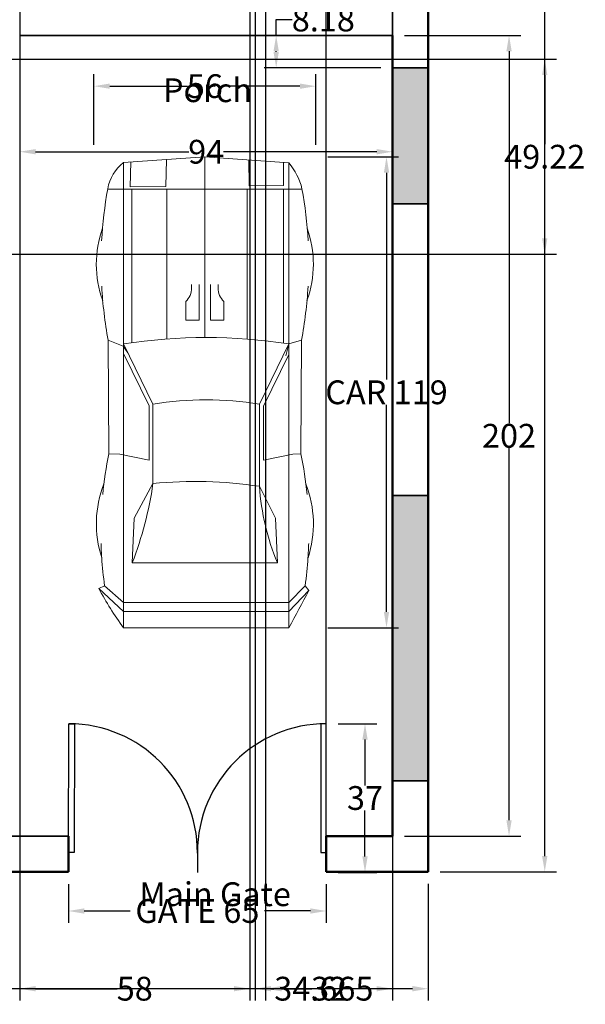
# Model space of a CAD drawing. Units: inches. Extents: x -1285 to -837, y -84 to 552.
# Tile 4 of 10: x -981 to -838, y -84 to 164. Entities that reach past the tile are written whole.
import ezdxf

# ---------------------------------------------------------------- set-up
doc = ezdxf.new("R2010")
doc.units = ezdxf.units.IN
doc.header["$MEASUREMENT"] = 0
for name, color, linetype, lineweight in [('A-ANNO-DIMS', 2, 'Continuous', 18), ('A-ANNO-TEXT', 7, 'Continuous', 18), ('A-AREA-IDEN', 7, 'Continuous', 25), ('A-COLS', 54, 'Continuous', 35), ('A-COLS-PATT', 54, 'Continuous', 13), ('Car', 10, 'Continuous', 18), ('Doors', 34, 'Continuous', 25), ('Inner Wall', 202, 'Continuous', 35), ('Outer Wall', 12, 'Continuous', 50)]:
    doc.layers.add(name, color=color, linetype=linetype, lineweight=lineweight)
doc.styles.get("Standard").update_dxf_attribs({"font": 'arial.ttf'})
doc.dimstyles.get("Standard").update_dxf_attribs({"dimtxt": 6, "dimasz": 4, "dimexe": 3, "dimexo": 3, "dimgap": 0.09, "dimtad": 0, "dimtih": 1, "dimtoh": 1, "dimdec": 1, "dimzin": 0, "dimdsep": 46, "dimlunit": 3, "dimtxsty": 'Standard', "dimcen": 0.09, "dimadec": 0, "dimazin": 0, "dimtfac": 1, "dimtdec": 1, "dimtofl": 0, "dimtmove": 0, "dimatfit": 3, "dimfxl": 1, "dimtolj": 1, "dimtzin": 0, "dimarcsym": 0})

# ---------------------------------------------------------------- blocks, each defined once
blk = doc.blocks.new('Car Top View')
for p, q in [((1583.58, 732.11), (1582.02, 730.88)), ((1587.49, 725.66), (1582.02, 730.88)), ((1590.39, 725.66), (1583.58, 732.11)), ((1454.09, 729.88), (1454.09, 667.25)), ((1504.06, 725.66), (1502.84, 729.72)), ((1502.84, 729.72), (1539.47, 729.51)), ((1539.64, 726.95), (1539.47, 729.51)), ((1443.7, 698.56), (1445.66, 725.66)), ((1595.59, 725.66), (1445.66, 725.66)), ((1504.06, 725.66), (1523.43, 716.14)), ((1507.93, 724.64), (1504.06, 725.66)), ((1507.44, 725.66), (1524.09, 717.48)), ((1541.57, 717.48), (1539.64, 726.95)), ((1587.49, 672.32), (1587.49, 725.66)), ((1590.39, 672.32), (1590.39, 725.66)), ((1595.59, 725.66), (1595.59, 672.32)), ((1445.53, 723.93), (1453, 723.93)), ((1453, 723.93), (1453.03, 712.83)), ((1454.09, 723.93), (1503.8, 723.93)), ((1549.96, 716.14), (1560.21, 721.31)), ((1560.21, 721.31), (1574.68, 721.97)), ((1574.68, 675.15), (1574.68, 721.97)), ((1523.43, 716.14), (1549.96, 716.14)), ((1524.09, 717.48), (1541.57, 717.48)), ((1453.03, 712.83), (1444.72, 712.69)), ((1454.09, 712.22), (1502.48, 712.22)), ((1484.93, 702.85), (1486.03, 702.85)), ((1496.41, 704.73), (1490.34, 704.73)), ((1496.41, 700.4), (1496.41, 704.73)), ((1484.93, 700.4), (1496.41, 700.4)), ((1443.7, 698.56), (1501.97, 698.56)), ((1443.7, 698.56), (1445.53, 672.32)), ((1484.93, 696.73), (1496.41, 696.73)), ((1496.41, 696.73), (1496.41, 692.4)), ((1484.93, 694.28), (1486.03, 694.28)), ((1496.41, 692.4), (1490.34, 692.4)), ((1453.3, 685.99), (1444.56, 686.18)), ((1453.4, 674.47), (1453.3, 685.99)), ((1454.09, 686.34), (1502.44, 686.34)), ((1504.06, 672.32), (1523.43, 681.84)), ((1507.1, 672.32), (1524.03, 680.64)), ((1523.43, 681.84), (1549.09, 681.84)), ((1524.03, 680.64), (1541.51, 680.64)), ((1541.51, 680.64), (1539.57, 671.17)), ((1549.09, 681.84), (1560.21, 675.82)), ((1445.36, 674.74), (1453.4, 674.47)), ((1454.09, 675.02), (1503.65, 675.02)), ((1506.89, 673.72), (1504.78, 672.2)), ((1560.21, 675.82), (1574.68, 675.15)), ((1445.53, 672.32), (1595.59, 672.32)), ((1504.78, 672.2), (1502.84, 667.41)), ((1539.57, 671.17), (1539.47, 667.62)), ((1587.49, 672.32), (1582.02, 666.25)), ((1590.39, 672.32), (1582.91, 664.38)), ((1502.84, 667.41), (1539.47, 667.62)), ((1582.91, 664.38), (1582.02, 666.25))]:
    blk.add_line(p, q)
for centre, radius, start, end in [((1478.3, 699.25), 34.3, 69.9626, 109.7406), ((1478.03, 596.84), 135.18, 93.0435, 100.2397), ((1478.03, 596.84), 135.18, 79.425, 86.8505), ((1564.7, 606.62), 125.46, 95.5274, 101.6043), ((1562.07, 698.12), 35.42, 72.0072, 111.2869), ((1564.7, 606.62), 125.46, 86.2021, 88.3127), ((1564.7, 606.62), 125.46, 82.0643, 86.2021), ((2098.75, 1676.59), 1075.84, 241.38974, 242.11561), ((1458.74, 710.05), 20.37, 103.473, 129.991), ((1673.24, 698.99), 171.27, 171.0429, 188.9571), ((1544.44, 794.77), 78.82, 274.0159, 292.5586), ((1630.35, 698.99), 108.28, 170.889, 189.111), ((1685.15, 695.55), 136.74, 171.3428, 185.7544), ((1486.11, 708.54), 5.7, 269.2285, 317.9431), ((1486.11, 688.58), 5.7, 42.0569, 90.7715), ((1531.58, 562.58), 120.54, 69.0476, 81.6444), ((1456.64, 681.32), 14.3, 218.99, 259.3637), ((1532.44, 759.05), 107.28, 298.064, 306.0621), ((1478.03, 800.29), 135.18, 259.7603, 266.9565), ((1478.03, 800.29), 135.18, 273.1495, 280.575), ((1564.7, 790.51), 125.46, 258.3957, 264.4726), ((1478.3, 697.88), 34.3, 250.2594, 290.0374), ((1562.07, 699.01), 35.42, 248.7131, 287.9928), ((1564.7, 790.51), 125.46, 271.6873, 273.7979), ((1564.7, 790.51), 125.46, 273.7979, 277.9357)]:
    blk.add_arc(centre, radius, start, end)
blk = doc.blocks.new('*U3')
for p, q in [((0, 0), (0, -6)), ((40, 0), (40, -6))]:
    blk.add_line(p, q)
blk.add_lwpolyline([(0, 0), (0, 40), (1.75, 40), (1.75, 0)], close=True)
blk.add_arc((0, 0), 40, 0, 90)
blk = doc.blocks.new('*U4')
for p, q in [((0, 0), (0, -6)), ((-40, 0), (-40, -6))]:
    blk.add_line(p, q)
blk.add_lwpolyline([(0, 0), (0, 40), (-1.75, 40), (-1.75, 0)], close=True)
blk.add_arc((0, 0), 40, 90, 180)
blk = doc.blocks.new('Main Gate')
at = {"xscale": 0.812505538442662, "yscale": 0.812505538442662, "zscale": 0.812505538442662, "rotation": 359.7884473139384}
blk.add_blockref('*U3', (1223.44, 655.96), dxfattribs=at)
at = {"xscale": 0.812500000000006, "yscale": 0.812500000000006, "zscale": 0.812500000000006}
blk.add_blockref('*U4', (1288.43, 655.96), dxfattribs=at)
blk = doc.blocks.new('WALL-PIER-34x9')
blk.add_lwpolyline([(9, 34.35), (9, 0), (0, 0), (0, 34.35)], close=True)
blk = doc.blocks.new('*D47')
at = {"layer": 'A-ANNO-DIMS', "color": 0, "lineweight": -2, "transparency": 16777216}
for p, q in [((-902.88, 129.31), (-885.07, 129.31)), ((-888.07, 125.31), (-888.07, 73.1)), ((-888.07, 14.51), (-888.07, 66.72)), ((-902.88, 10.51), (-885.07, 10.51))]:
    blk.add_line(p, q, dxfattribs=at)
at = {"layer": 'A-ANNO-DIMS', "color": 0, "transparency": 16777216}
for points in [[(-888.73, 125.31), (-887.4, 125.31), (-888.07, 129.31)], [(-888.73, 14.51), (-887.4, 14.51), (-888.07, 10.51)]]:
    blk.add_solid(points, dxfattribs=at)
at = {"layer": 'Defpoints', "color": 0, "transparency": 16777216}
for p in [(-905.88, 129.31), (-905.88, 10.51), (-888.07, 10.51)]:
    blk.add_point(p, dxfattribs=at)
at = {"layer": 'A-ANNO-DIMS', "color": 0, "transparency": 16777216, "insert": (-888.07, 69.91), "char_height": 6, "attachment_point": 5}
blk.add_mtext('\\A1;CAR 119', dxfattribs=at)
blk = doc.blocks.new('*D48')
at = {"layer": 'A-ANNO-DIMS', "color": 0, "lineweight": -2, "transparency": 16777216}
for p, q in [((-961.83, 132.31), (-961.83, 150.13)), ((-905.88, 132.31), (-905.88, 150.13)), ((-957.83, 147.13), (-938.24, 147.13)), ((-909.88, 147.13), (-929.47, 147.13))]:
    blk.add_line(p, q, dxfattribs=at)
at = {"layer": 'A-ANNO-DIMS', "color": 0, "transparency": 16777216}
for points in [[(-957.83, 147.79), (-957.83, 146.46), (-961.83, 147.13)], [(-909.88, 147.79), (-909.88, 146.46), (-905.88, 147.13)]]:
    blk.add_solid(points, dxfattribs=at)
at = {"layer": 'Defpoints', "color": 0, "transparency": 16777216}
for p in [(-905.88, 147.13), (-961.83, 129.31), (-905.88, 129.31)]:
    blk.add_point(p, dxfattribs=at)
at = {"layer": 'A-ANNO-DIMS', "color": 0, "transparency": 16777216, "insert": (-933.86, 147.13), "char_height": 6, "attachment_point": 5}
blk.add_mtext('\\A1;56', dxfattribs=at)
blk = doc.blocks.new('*D63')
at = {"layer": 'A-ANNO-DIMS', "color": 0, "lineweight": -2, "transparency": 16777216}
for p, q in [((-968.24, -54.18), (-968.24, -63.93)), ((-903.24, -54.18), (-903.24, -63.93)), ((-964.24, -60.93), (-952.68, -60.93)), ((-907.24, -60.93), (-918.8, -60.93))]:
    blk.add_line(p, q, dxfattribs=at)
at = {"layer": 'A-ANNO-DIMS', "color": 0, "transparency": 16777216}
for points in [[(-964.24, -60.26), (-964.24, -61.6), (-968.24, -60.93)], [(-907.24, -60.26), (-907.24, -61.6), (-903.24, -60.93)]]:
    blk.add_solid(points, dxfattribs=at)
at = {"layer": 'Defpoints', "color": 0, "transparency": 16777216}
for p in [(-968.24, -51.18), (-903.24, -51.18), (-903.24, -60.93)]:
    blk.add_point(p, dxfattribs=at)
at = {"layer": 'A-ANNO-DIMS', "color": 0, "transparency": 16777216, "insert": (-935.74, -60.93), "char_height": 6, "attachment_point": 5}
blk.add_mtext('\\A1;GATE 65', dxfattribs=at)
blk = doc.blocks.new('*D64')
at = {"layer": 'A-ANNO-DIMS', "color": 0, "lineweight": -2, "transparency": 16777216}
for p, q in [((-900.24, -13.69), (-890.49, -13.69)), ((-893.49, -17.69), (-893.49, -29.28)), ((-893.49, -47.18), (-893.49, -35.59)), ((-900.24, -51.18), (-890.49, -51.18))]:
    blk.add_line(p, q, dxfattribs=at)
at = {"layer": 'A-ANNO-DIMS', "color": 0, "transparency": 16777216}
for points in [[(-894.16, -17.69), (-892.82, -17.69), (-893.49, -13.69)], [(-894.16, -47.18), (-892.82, -47.18), (-893.49, -51.18)]]:
    blk.add_solid(points, dxfattribs=at)
at = {"layer": 'Defpoints', "color": 0, "transparency": 16777216}
for p in [(-903.24, -13.69), (-893.49, -13.69), (-903.24, -51.18)]:
    blk.add_point(p, dxfattribs=at)
at = {"layer": 'A-ANNO-DIMS', "color": 0, "transparency": 16777216, "insert": (-893.49, -32.43), "char_height": 6, "attachment_point": 5}
blk.add_mtext('\\A1;37', dxfattribs=at)
blk = doc.blocks.new('*D69')
at = {"layer": 'A-ANNO-DIMS', "color": 0, "lineweight": -2, "transparency": 16777216}
for p, q in [((-1245.53, -54.06), (-1245.53, -83.53)), ((-877.53, -54.06), (-877.53, -83.53)), ((-1241.53, -80.53), (-1068.25, -80.53)), ((-881.53, -80.53), (-1054.81, -80.53))]:
    blk.add_line(p, q, dxfattribs=at)
at = {"layer": 'A-ANNO-DIMS', "color": 0, "transparency": 16777216}
for points in [[(-1241.53, -79.86), (-1241.53, -81.2), (-1245.53, -80.53)], [(-881.53, -79.86), (-881.53, -81.2), (-877.53, -80.53)]]:
    blk.add_solid(points, dxfattribs=at)
at = {"layer": 'Defpoints', "color": 0, "transparency": 16777216}
for p in [(-1245.53, -51.06), (-877.53, -51.06), (-877.53, -80.53)]:
    blk.add_point(p, dxfattribs=at)
at = {"layer": 'A-ANNO-DIMS', "color": 0, "transparency": 16777216, "insert": (-1061.53, -80.53), "char_height": 6, "attachment_point": 5}
blk.add_mtext('\\A1;368', dxfattribs=at)
blk = doc.blocks.new('*D70')
at = {"layer": 'A-ANNO-DIMS', "color": 0, "lineweight": -2, "transparency": 16777216}
for p, q in [((-874.53, 518.94), (-845.18, 518.94)), ((-848.18, 514.94), (-848.18, 237.09)), ((-848.18, -47.06), (-848.18, 230.79)), ((-874.53, -51.06), (-845.18, -51.06))]:
    blk.add_line(p, q, dxfattribs=at)
at = {"layer": 'A-ANNO-DIMS', "color": 0, "transparency": 16777216}
for points in [[(-848.85, 514.94), (-847.51, 514.94), (-848.18, 518.94)], [(-848.85, -47.06), (-847.51, -47.06), (-848.18, -51.06)]]:
    blk.add_solid(points, dxfattribs=at)
at = {"layer": 'Defpoints', "color": 0, "transparency": 16777216}
for p in [(-877.53, 518.94), (-848.18, 518.94), (-877.53, -51.06)]:
    blk.add_point(p, dxfattribs=at)
at = {"layer": 'A-ANNO-DIMS', "color": 0, "transparency": 16777216, "insert": (-848.18, 233.94), "char_height": 6, "attachment_point": 5}
blk.add_mtext('\\A1;570', dxfattribs=at)
blk = doc.blocks.new('*D81')
at = {"layer": 'A-ANNO-DIMS', "color": 0, "lineweight": -2, "transparency": 16777216}
for p, q in [((-980.53, 156.94), (-980.53, 127.59)), ((-886.53, 156.94), (-886.53, 127.59)), ((-976.53, 130.59), (-937.9, 130.59)), ((-890.53, 130.59), (-929.15, 130.59))]:
    blk.add_line(p, q, dxfattribs=at)
at = {"layer": 'A-ANNO-DIMS', "color": 0, "transparency": 16777216}
for points in [[(-976.53, 131.26), (-976.53, 129.92), (-980.53, 130.59)], [(-890.53, 131.26), (-890.53, 129.92), (-886.53, 130.59)]]:
    blk.add_solid(points, dxfattribs=at)
at = {"layer": 'Defpoints', "color": 0, "transparency": 16777216}
for p in [(-980.53, 159.94), (-886.53, 159.94), (-980.53, 130.59)]:
    blk.add_point(p, dxfattribs=at)
at = {"layer": 'A-ANNO-DIMS', "color": 0, "transparency": 16777216, "insert": (-933.53, 130.59), "char_height": 6, "attachment_point": 5}
blk.add_mtext('\\A1;94', dxfattribs=at)
blk = doc.blocks.new('*D85')
at = {"layer": 'A-ANNO-DIMS', "color": 0, "lineweight": -2, "transparency": 16777216}
for p, q in [((-980.53, 310.94), (-980.53, -83.53)), ((-922.53, 310.94), (-922.53, -83.53)), ((-976.53, -80.53), (-955.92, -80.53)), ((-926.53, -80.53), (-947.14, -80.53))]:
    blk.add_line(p, q, dxfattribs=at)
at = {"layer": 'A-ANNO-DIMS', "color": 0, "transparency": 16777216}
for points in [[(-976.53, -79.86), (-976.53, -81.2), (-980.53, -80.53)], [(-926.53, -79.86), (-926.53, -81.2), (-922.53, -80.53)]]:
    blk.add_solid(points, dxfattribs=at)
at = {"layer": 'Defpoints', "color": 0, "transparency": 16777216}
for p in [(-980.53, 313.94), (-922.53, 313.94), (-922.53, -80.53)]:
    blk.add_point(p, dxfattribs=at)
at = {"layer": 'A-ANNO-DIMS', "color": 0, "transparency": 16777216, "insert": (-951.53, -80.53), "char_height": 6, "attachment_point": 5}
blk.add_mtext('\\A1;58', dxfattribs=at)
blk = doc.blocks.new('*D86')
at = {"layer": 'A-ANNO-DIMS', "color": 0, "lineweight": -2, "transparency": 16777216}
for p, q in [((-918.53, 310.94), (-918.53, -83.53)), ((-886.53, 310.94), (-886.53, -83.53)), ((-914.53, -80.53), (-906.88, -80.53)), ((-890.53, -80.53), (-898.18, -80.53))]:
    blk.add_line(p, q, dxfattribs=at)
at = {"layer": 'A-ANNO-DIMS', "color": 0, "transparency": 16777216}
for points in [[(-914.53, -79.86), (-914.53, -81.2), (-918.53, -80.53)], [(-890.53, -79.86), (-890.53, -81.2), (-886.53, -80.53)]]:
    blk.add_solid(points, dxfattribs=at)
at = {"layer": 'Defpoints', "color": 0, "transparency": 16777216}
for p in [(-918.53, 313.94), (-886.53, 313.94), (-886.53, -80.53)]:
    blk.add_point(p, dxfattribs=at)
at = {"layer": 'A-ANNO-DIMS', "color": 0, "transparency": 16777216, "insert": (-902.53, -80.53), "char_height": 6, "attachment_point": 5}
blk.add_mtext('\\A1;32', dxfattribs=at)
blk = doc.blocks.new('*D92')
at = {"layer": 'A-ANNO-DIMS', "color": 0, "lineweight": -2, "transparency": 16777216}
for p, q in [((-1113.53, 153.94), (-845.18, 153.94)), ((-848.18, 149.94), (-848.18, 132.48)), ((-848.18, 108.72), (-848.18, 126.18)), ((-1113.53, 104.72), (-845.18, 104.72))]:
    blk.add_line(p, q, dxfattribs=at)
at = {"layer": 'A-ANNO-DIMS', "color": 0, "transparency": 16777216}
for points in [[(-848.85, 149.94), (-847.51, 149.94), (-848.18, 153.94)], [(-848.85, 108.72), (-847.51, 108.72), (-848.18, 104.72)]]:
    blk.add_solid(points, dxfattribs=at)
at = {"layer": 'Defpoints', "color": 0, "transparency": 16777216}
for p in [(-1116.53, 153.94), (-848.18, 153.94), (-1116.53, 104.72)]:
    blk.add_point(p, dxfattribs=at)
at = {"layer": 'A-ANNO-DIMS', "color": 0, "transparency": 16777216, "insert": (-848.18, 129.33), "char_height": 6, "attachment_point": 5}
blk.add_mtext('\\A1;49.22', dxfattribs=at)
blk = doc.blocks.new('*D97')
at = {"layer": 'A-ANNO-DIMS', "color": 0, "lineweight": -2, "transparency": 16777216}
for p, q in [((-921.19, 506.94), (-921.19, -83.53)), ((-886.53, 506.94), (-886.53, -83.53)), ((-917.19, -80.53), (-916.43, -80.53)), ((-890.53, -80.53), (-891.3, -80.53))]:
    blk.add_line(p, q, dxfattribs=at)
at = {"layer": 'A-ANNO-DIMS', "color": 0, "transparency": 16777216}
for points in [[(-917.19, -79.86), (-917.19, -81.2), (-921.19, -80.53)], [(-890.53, -79.86), (-890.53, -81.2), (-886.53, -80.53)]]:
    blk.add_solid(points, dxfattribs=at)
at = {"layer": 'Defpoints', "color": 0, "transparency": 16777216}
for p in [(-921.19, 509.94), (-886.53, 509.94), (-886.53, -80.53)]:
    blk.add_point(p, dxfattribs=at)
at = {"layer": 'A-ANNO-DIMS', "color": 0, "transparency": 16777216, "insert": (-903.86, -80.53), "char_height": 6, "attachment_point": 5}
blk.add_mtext('\\A1;34.665', dxfattribs=at)
blk = doc.blocks.new('*D102')
at = {"layer": 'A-ANNO-DIMS', "color": 0, "lineweight": -2, "transparency": 16777216}
for p, q in [((-903.24, -39.06), (-903.24, 551.29)), ((-886.53, -39.06), (-886.53, 551.29)), ((-899.24, 548.29), (-890.53, 548.29)), ((-886.53, 548.29), (-882.53, 548.29))]:
    blk.add_line(p, q, dxfattribs=at)
at = {"layer": 'A-ANNO-DIMS', "color": 0, "transparency": 16777216}
for points in [[(-899.24, 548.96), (-899.24, 547.62), (-903.24, 548.29)], [(-890.53, 548.96), (-890.53, 547.62), (-886.53, 548.29)]]:
    blk.add_solid(points, dxfattribs=at)
at = {"layer": 'Defpoints', "color": 0, "transparency": 16777216}
for p in [(-886.53, 548.29), (-903.24, -42.06), (-886.53, -42.06)]:
    blk.add_point(p, dxfattribs=at)
at = {"layer": 'A-ANNO-DIMS', "color": 0, "transparency": 16777216, "insert": (-873.18, 548.29), "char_height": 6, "attachment_point": 5}
blk.add_mtext('\\A1;16.71', dxfattribs=at)
blk = doc.blocks.new('*D109')
at = {"layer": 'A-ANNO-DIMS', "color": 0, "lineweight": -2, "transparency": 16777216}
for p, q in [((-883.53, 159.94), (-854.18, 159.94)), ((-857.18, 155.94), (-857.18, 62.09)), ((-857.18, -38.06), (-857.18, 55.79)), ((-883.53, -42.06), (-854.18, -42.06))]:
    blk.add_line(p, q, dxfattribs=at)
at = {"layer": 'A-ANNO-DIMS', "color": 0, "transparency": 16777216}
for points in [[(-857.85, 155.94), (-856.51, 155.94), (-857.18, 159.94)], [(-857.85, -38.06), (-856.51, -38.06), (-857.18, -42.06)]]:
    blk.add_solid(points, dxfattribs=at)
at = {"layer": 'Defpoints', "color": 0, "transparency": 16777216}
for p in [(-886.53, 159.94), (-886.53, -42.06), (-857.18, -42.06)]:
    blk.add_point(p, dxfattribs=at)
at = {"layer": 'A-ANNO-DIMS', "color": 0, "transparency": 16777216, "insert": (-857.18, 58.94), "char_height": 6, "attachment_point": 5}
blk.add_mtext('\\A1;202', dxfattribs=at)
blk = doc.blocks.new('*D114')
at = {"layer": 'A-ANNO-DIMS', "color": 0, "lineweight": -2, "transparency": 16777216}
for p, q in [((-915.88, 159.94), (-915.88, 163.94)), ((-915.88, 163.94), (-911.88, 163.94)), ((-889.53, 159.94), (-918.88, 159.94)), ((-915.88, 155.76), (-915.88, 155.94)), ((-889.53, 151.76), (-918.88, 151.76))]:
    blk.add_line(p, q, dxfattribs=at)
at = {"layer": 'A-ANNO-DIMS', "color": 0, "transparency": 16777216}
for points in [[(-916.55, 155.94), (-915.21, 155.94), (-915.88, 159.94)], [(-916.55, 155.76), (-915.21, 155.76), (-915.88, 151.76)]]:
    blk.add_solid(points, dxfattribs=at)
at = {"layer": 'Defpoints', "color": 0, "transparency": 16777216}
for p in [(-915.88, 159.94), (-886.53, 159.94), (-886.53, 151.76)]:
    blk.add_point(p, dxfattribs=at)
at = {"layer": 'A-ANNO-DIMS', "color": 0, "transparency": 16777216, "insert": (-903.99, 163.94), "char_height": 6, "attachment_point": 5}
blk.add_mtext('\\A1;8.18', dxfattribs=at)

msp = doc.modelspace()

# ---------------------------------------------------------------- hatches: boundary and pattern name
at = {"layer": 'A-COLS-PATT'}
h = msp.add_hatch(color=256, dxfattribs=at)
h.dxf.hatch_style = 1
h.paths.add_polyline_path([(-1236.5299, 354.7957), (-1245.5299, 354.7957), (-1245.5299, 320.4471), (-1236.5299, 320.4471)])
h.paths.add_polyline_path([(-1236.5299, 466.4307), (-1245.5299, 466.4307), (-1245.5299, 432.0821), (-1236.5299, 432.0821)])
h.paths.add_polyline_path([(-877.5299, 151.7586), (-886.5299, 151.7586), (-886.5299, 117.41), (-877.5299, 117.41)])
h.paths.add_polyline_path([(-877.5299, 43.9103), (-886.5299, 43.9103), (-886.5299, -28.0897), (-877.5299, -28.0897)])
h.paths.add_polyline_path([(-1236.5299, 203.7523), (-1245.5299, 203.7523), (-1245.5299, 169.4036), (-1236.5299, 169.4036)])

# ---------------------------------------------------------------- linework, layer by layer
at = {"layer": 'A-COLS'}
msp.add_lwpolyline([(-877.5299, 43.9103), (-877.5299, -28.0897), (-886.5299, -28.0897), (-886.5299, 43.9103)], close=True, dxfattribs=at)
at = {"layer": 'Doors'}
for p, q in [((-935.7229, -46.5608), (-935.74, -46.5608)), ((-935.74, -51.0608), (-935.74, -51.1808)), ((-935.74, -51.0608), (-935.7396, -51.0608))]:
    msp.add_line(p, q, dxfattribs=at)
at = {"layer": 'Inner Wall'}
msp.add_line((-980.5299, 159.9392), (-886.5299, 159.9392), dxfattribs=at)
msp.add_lwpolyline([(-1028.5299, 75.9392), (-1028.5299, -42.0608), (-968.24, -42.0608)], dxfattribs=at)
at = {"layer": 'Outer Wall'}
for p, q in [((-877.5299, 518.9392), (-877.5299, -51.0608)), ((-886.5299, 159.9392), (-886.5299, -42.0608)), ((-968.24, -42.0608), (-968.24, -51.0608)), ((-903.24, -42.0608), (-903.24, -51.0608)), ((-903.24, -42.0608), (-886.5299, -42.0608)), ((-1245.5299, -51.0608), (-968.24, -51.0608)), ((-903.24, -51.0608), (-877.5299, -51.0608))]:
    msp.add_line(p, q, dxfattribs=at)

# ---------------------------------------------------------------- block references
at = {"layer": 'A-COLS'}
msp.add_blockref('WALL-PIER-34x9', (-886.53, 117.4099), dxfattribs=at)
at = {"layer": 'Car', "xscale": 0.782135332514792, "yscale": 0.782135332514792, "zscale": 0.782135332514792, "rotation": 270}
msp.add_blockref('Car Top View', (-1480.2279, 1258.4807), dxfattribs=at)
at = {"layer": 'Doors'}
msp.add_blockref('Main Gate', (-2191.666, -702.1458), dxfattribs=at)

# ---------------------------------------------------------------- texts
at = {"layer": 'A-ANNO-TEXT', "insert": (-965.6734, -53.6991), "char_height": 6, "attachment_point": 1}
msp.add_mtext_dynamic_manual_height_columns('\\pxqc;Main Gate', width=68.784729, gutter_width=1, heights=[0], dxfattribs=at)
at = {"layer": 'A-AREA-IDEN', "insert": (-967.5873, 149.104), "char_height": 6, "attachment_point": 1}
msp.add_mtext_dynamic_manual_height_columns('\\pxqc;Porch', width=68.784729, gutter_width=1, heights=[0], dxfattribs=at)

# ---------------------------------------------------------------- dimensions: what is measured, and where the dimension line sits
at = {"layer": 'A-ANNO-DIMS'}
for base, p1, p2, override, picture, middle in [((-886.5299, 548.2892), (-903.24, -42.0608), (-886.5299, -42.0608), {"dimdec": 2, "dimlfac": 1, "dimrnd": 0, "dimzin": 0, "dimdsep": 46, "dimlunit": 2}, '*D102', (-873.1779, 548.2892)), ((-886.5299, -80.5308), (-921.1945, 509.9392), (-886.5299, 509.9392), {"dimdec": 3, "dimlfac": 1, "dimrnd": 0, "dimzin": 0, "dimdsep": 46, "dimlunit": 2}, '*D97', (-903.8622, -80.5308)), ((-922.5299, -80.5308), (-980.5299, 313.9392), (-922.5299, 313.9392), {"dimdec": 0, "dimlfac": 1, "dimrnd": 0, "dimzin": 0, "dimdsep": 46, "dimlunit": 2}, '*D85', (-951.5299, -80.5308)), ((-886.5299, -80.5308), (-918.5299, 313.9392), (-886.5299, 313.9392), {"dimdec": 0, "dimlfac": 1, "dimrnd": 0, "dimzin": 0, "dimdsep": 46, "dimlunit": 2}, '*D86', (-902.5299, -80.5308)), ((-905.8846, 147.1274), (-961.8275, 129.3083), (-905.8846, 129.3083), {"dimdec": 0, "dimlfac": 1, "dimrnd": 0, "dimzin": 0, "dimdsep": 46, "dimlunit": 2}, '*D48', (-933.8561, 147.1274)), ((-877.5299, -80.5308), (-1245.5299, -51.0608), (-877.5299, -51.0608), {"dimdec": 0, "dimlfac": 1, "dimrnd": 0, "dimzin": 0, "dimdsep": 46, "dimlunit": 2}, '*D69', (-1061.5299, -80.5308))]:
    dim = msp.add_linear_dim(base=base, p1=p1, p2=p2, dimstyle='Standard', override=override, dxfattribs=at)
    dim.commit()
    dim.dimension.update_dxf_attribs({"geometry": picture, "text_midpoint": middle})
for base, p1, p2, angle, override, picture, middle in [((-848.1799, 518.9392), (-877.5299, -51.0608), (-877.5299, 518.9392), 90, {"dimdec": 0, "dimlfac": 1, "dimrnd": 0, "dimzin": 0, "dimdsep": 46, "dimlunit": 2}, '*D70', (-848.1799, 233.9392)), ((-915.8799, 159.9392), (-886.5299, 151.7586), (-886.5299, 159.9392), 90, {"dimdec": 2, "dimlfac": 1, "dimrnd": 0, "dimzin": 0, "dimdsep": 46, "dimlunit": 2}, '*D114', (-903.987, 163.9392)), ((-980.5299, 130.5892), (-886.5299, 159.9392), (-980.5299, 159.9392), 180, {"dimdec": 0, "dimlfac": 1, "dimrnd": 0, "dimzin": 0, "dimdsep": 46, "dimlunit": 2}, '*D81', (-933.5299, 130.5892)), ((-857.1799, -42.0608), (-886.5299, 159.9392), (-886.5299, -42.0608), 270, {"dimdec": 0, "dimlfac": 1, "dimrnd": 0, "dimzin": 0, "dimdsep": 46, "dimlunit": 2}, '*D109', (-857.1799, 58.9392)), ((-848.1799, 153.9392), (-1116.5299, 104.7212), (-1116.5299, 153.9392), 90, {"dimdec": 2, "dimlfac": 1, "dimrnd": 0, "dimzin": 0, "dimdsep": 46, "dimlunit": 2}, '*D92', (-848.1799, 129.3302)), ((-893.49, -13.6858), (-903.24, -51.1808), (-903.24, -13.6858), 90, {"dimdec": 0, "dimlfac": 1, "dimrnd": 0, "dimzin": 0, "dimdsep": 46, "dimlunit": 2}, '*D64', (-893.49, -32.4333))]:
    dim = msp.add_linear_dim(base=base, p1=p1, p2=p2, angle=angle, dimstyle='Standard', override=override, dxfattribs=at)
    dim.commit()
    dim.dimension.update_dxf_attribs({"geometry": picture, "text_midpoint": middle})
dim = msp.add_linear_dim(base=(-888.0655, 10.5144), p1=(-905.8846, 129.3083), p2=(-905.8846, 10.5144), angle=270, text='CAR <>', dimstyle='Standard', override={"dimdec": 0, "dimlfac": 1, "dimrnd": 0, "dimzin": 0, "dimdsep": 46, "dimlunit": 2}, dxfattribs=at)
dim.commit()
dim.dimension.update_dxf_attribs({"geometry": '*D47', "text_midpoint": (-888.0655, 69.9114)})
dim = msp.add_linear_dim(base=(-903.24, -60.9308), p1=(-968.24, -51.1808), p2=(-903.24, -51.1808), text='GATE <>', dimstyle='Standard', override={"dimdec": 0, "dimlfac": 1, "dimrnd": 0, "dimzin": 0, "dimdsep": 46, "dimlunit": 2}, dxfattribs=at)
dim.commit()
dim.dimension.update_dxf_attribs({"geometry": '*D63', "text_midpoint": (-935.74, -60.9308)})

doc.saveas('drawing.dxf')
